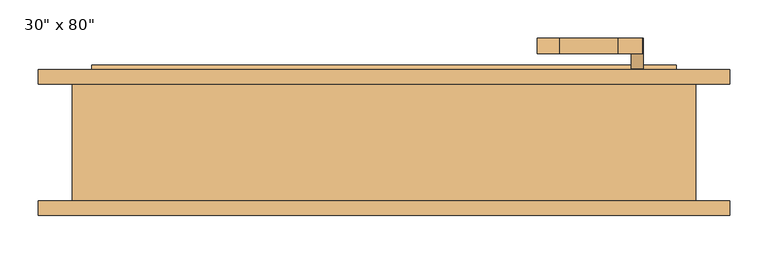
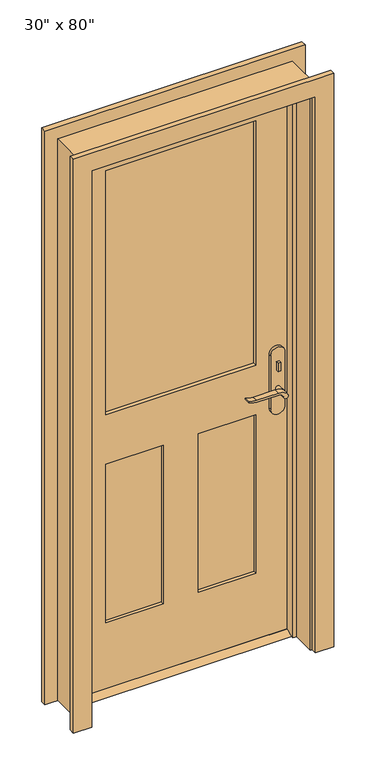
"""IFC4 building model written with IfcOpenShell, lengths in millimetres: door geometry."""

from ifc_helpers import new_model, si_unit, point, frame, frame_2d, origin, place, context, project, spatial, polyline, circle_curve, trimmed, segment, composite_curve, outline, extrude, faceted_brep, source, transform, mapped, element, save


def door_cdf9d6cc(model_context):
    return source(origin(), model_context, "Body", "SolidModel", [
        extrude(outline(polyline([(38.1, 12.7), (73.025, 12.7), (98.425, 0.0), (12.7, 0.0), (38.1, 12.7)])), frame((-381.0, 0.0, 0.0), z_axis=(1.0, 0.0, 0.0), x_axis=(0.0, 1.0, 0.0)), (0.0, 0.0, 1.0), 762.0),
        extrude(outline(polyline([(335.2, 18.1), (325.2, 18.1), (325.2, 28.1), (335.2, 28.1), (335.2, 18.1)])), frame((0.0, 0.0, 981.9), z_axis=(0.0, 0.0, 1.0), x_axis=(1.0, 0.0, 0.0)), (0.0, 0.0, 1.0), 30.0),
        extrude(outline(composite_curve([segment(trimmed(circle_curve(frame_2d((996.9, 330.2)), 8.0), [point((996.9, 322.2))], [point((996.9, 338.2))], False, "CARTESIAN"), True, "CONTINUOUS"), segment(trimmed(circle_curve(frame_2d((996.9, 330.2)), 8.0), [point((996.9, 338.2))], [point((996.9, 322.2))], False, "CARTESIAN"), True, "CONTINUOUS")], self_intersect=False)), frame((0.0, 83.025, 0.0), z_axis=(0.0, 1.0, 0.0), x_axis=(0.0, 0.0, 1.0)), (0.0, 0.0, 1.0), 10.0),
        extrude(outline(composite_curve([segment(trimmed(circle_curve(frame_2d((897.1555521, 306.5324871)), 37.2832219), [point((919.0523287, 336.7081363))], [point((934.4, 304.8325667))], False, "CARTESIAN"), True, "CONTINUOUS"), segment(polyline([(934.4, 304.8325667), (934.4, 228.5564091)]), True, "CONTINUOUS"), segment(trimmed(circle_curve(frame_2d((1017.6850638, 228.6227909)), 83.2850902), [point((934.4, 228.5564091))], [point((939.4, 200.2))], True, "CARTESIAN"), True, "CONTINUOUS"), segment(polyline([(939.4, 200.2), (936.6135558, 200.2)]), True, "CONTINUOUS"), segment(trimmed(circle_curve(frame_2d((986.6709207, 232.1396612)), 59.3791355), [point((936.6135558, 200.2))], [point((927.4, 228.5564091))], False, "CARTESIAN"), True, "CONTINUOUS"), segment(polyline([(927.4, 228.5564091), (927.4, 304.8138099)]), True, "CONTINUOUS"), segment(trimmed(circle_curve(frame_2d((909.2738613, 304.8138099)), 18.1261387), [point((927.4, 304.8138099))], [point((914.4, 322.2))], True, "CARTESIAN"), True, "CONTINUOUS"), segment(trimmed(circle_curve(frame_2d((914.4, 330.2)), 8.0), [point((914.4, 322.2))], [point((919.0523287, 336.7081363))], False, "CARTESIAN"), True, "CONTINUOUS")], self_intersect=False)), frame((0.0, -21.9, 0.0), z_axis=(0.0, 1.0, 0.0), x_axis=(0.0, 0.0, 1.0)), (0.0, 0.0, 1.0), 20.0),
        extrude(outline(composite_curve([segment(trimmed(circle_curve(frame_2d((914.4, 330.2)), 8.0), [point((914.3999903, 322.2))], [point((919.0523287, 336.7081363))], False, "CARTESIAN"), True, "CONTINUOUS"), segment(trimmed(circle_curve(frame_2d((897.1555521, 306.5324871)), 37.2832219), [point((919.0523287, 336.7081363))], [point((934.4, 304.8325667))], False, "CARTESIAN"), True, "CONTINUOUS"), segment(polyline([(934.4, 304.8325667), (934.4, 228.5564091)]), True, "CONTINUOUS"), segment(trimmed(circle_curve(frame_2d((1017.6850638, 228.6227909)), 83.2850902), [point((934.4, 228.5564091))], [point((939.4, 200.2))], True, "CARTESIAN"), True, "CONTINUOUS"), segment(polyline([(939.4, 200.2), (936.6135558, 200.2)]), True, "CONTINUOUS"), segment(trimmed(circle_curve(frame_2d((986.6709207, 232.1396612)), 59.3791355), [point((936.6135558, 200.2))], [point((927.4, 228.5564091))], False, "CARTESIAN"), True, "CONTINUOUS"), segment(polyline([(927.4, 228.5564091), (927.4, 304.8138122)]), True, "CONTINUOUS"), segment(trimmed(circle_curve(frame_2d((909.2738682, 304.8138122)), 18.1261318), [point((927.4, 304.8138122))], [point((914.3999903, 322.2))], True, "CARTESIAN"), True, "CONTINUOUS")], self_intersect=False)), frame((0.0, 113.025, 0.0), z_axis=(0.0, 1.0, 0.0), x_axis=(0.0, 0.0, 1.0)), (0.0, 0.0, 1.0), 20.0),
        extrude(outline(composite_curve([segment(trimmed(circle_curve(frame_2d((914.4, 330.2)), 8.0), [point((914.4, 322.2))], [point((914.4, 338.2))], False, "CARTESIAN"), True, "CONTINUOUS"), segment(trimmed(circle_curve(frame_2d((914.4, 330.2)), 8.0), [point((914.4, 338.2))], [point((914.4, 322.2))], False, "CARTESIAN"), True, "CONTINUOUS")], self_intersect=False)), frame((0.0, -1.9, 0.0), z_axis=(0.0, 1.0, 0.0), x_axis=(0.0, 0.0, 1.0)), (0.0, 0.0, 1.0), 30.0),
        extrude(outline(composite_curve([segment(trimmed(circle_curve(frame_2d((914.4, 330.2)), 8.0), [point((914.4, 322.2))], [point((914.4, 338.2))], False, "CARTESIAN"), True, "CONTINUOUS"), segment(trimmed(circle_curve(frame_2d((914.4, 330.2)), 8.0), [point((914.4, 338.2))], [point((914.4, 322.2))], False, "CARTESIAN"), True, "CONTINUOUS")], self_intersect=False)), frame((0.0, 83.025, 0.0), z_axis=(0.0, 1.0, 0.0), x_axis=(0.0, 0.0, 1.0)), (0.0, 0.0, 1.0), 30.0),
        extrude(outline(composite_curve([segment(polyline([(844.4, 355.2), (1039.4, 355.2)]), True, "CONTINUOUS"), segment(trimmed(circle_curve(frame_2d((1039.4, 330.2)), 25.0), [point((1039.4, 355.2))], [point((1039.4, 305.2))], False, "CARTESIAN"), True, "CONTINUOUS"), segment(polyline([(1039.4, 305.2), (844.4, 305.2)]), True, "CONTINUOUS"), segment(trimmed(circle_curve(frame_2d((844.4, 330.2)), 25.0), [point((844.4, 305.2))], [point((844.4, 355.2))], False, "CARTESIAN"), True, "CONTINUOUS")], self_intersect=False)), frame((0.0, 28.1, 0.0), z_axis=(0.0, 1.0, 0.0), x_axis=(0.0, 0.0, 1.0)), (0.0, 0.0, 1.0), 10.0),
        extrude(outline(composite_curve([segment(polyline([(844.4, 355.2), (1039.4, 355.2)]), True, "CONTINUOUS"), segment(trimmed(circle_curve(frame_2d((1039.4, 330.2)), 25.0), [point((1039.4, 355.2))], [point((1039.4, 305.2))], False, "CARTESIAN"), True, "CONTINUOUS"), segment(polyline([(1039.4, 305.2), (844.4, 305.2)]), True, "CONTINUOUS"), segment(trimmed(circle_curve(frame_2d((844.4, 330.2)), 25.0), [point((844.4, 305.2))], [point((844.4, 355.2))], False, "CARTESIAN"), True, "CONTINUOUS")], self_intersect=False)), frame((0.0, 73.025, 0.0), z_axis=(0.0, 1.0, 0.0), x_axis=(0.0, 0.0, 1.0)), (0.0, 0.0, 1.0), 10.0),
        extrude(outline(polyline([(2032.0, -381.0), (12.7, -381.0), (12.7, 381.0), (2032.0, 381.0), (2032.0, -381.0)]), holes=[polyline([(1016.0, -260.35), (1911.35, -260.35), (1911.35, 260.35), (1016.0, 260.35), (1016.0, -260.35)]), polyline([(835.025, -60.325), (254.0, -60.325), (254.0, -260.35), (835.025, -260.35), (835.025, -60.325)]), polyline([(835.025, 260.35), (254.0, 260.35), (254.0, 60.325), (835.025, 60.325), (835.025, 260.35)])]), frame((0.0, 38.1, 0.0), z_axis=(0.0, 1.0, 0.0), x_axis=(0.0, 0.0, 1.0)), (0.0, 0.0, 1.0), 34.925),
        faceted_brep([(406.4, 73.025, 0.0), (406.4, -79.375, 0.0), (381.0, -79.375, 0.0), (381.0, 3.175, 0.0), (368.3, 3.175, 0.0), (368.3, 38.1, 0.0), (381.0, 38.1, 0.0), (381.0, 73.025, 0.0), (406.4, 73.025, 2057.4), (406.4, -79.375, 2057.4), (-406.4, -79.375, 2057.4), (-406.4, -79.375, 0.0), (-381.0, -79.375, 0.0), (-381.0, -79.375, 2032.0), (381.0, -79.375, 2032.0), (381.0, 3.175, 2032.0), (-381.0, 3.175, 2032.0), (-381.0, 3.175, 0.0), (-368.3, 3.175, 0.0), (-368.3, 3.175, 2019.3), (368.3, 3.175, 2019.3), (368.3, 38.1, 2019.3), (-368.3, 38.1, 2019.3), (-368.3, 38.1, 0.0), (-381.0, 38.1, 0.0), (-381.0, 38.1, 2032.0), (381.0, 38.1, 2032.0), (381.0, 73.025, 2032.0), (-381.0, 73.025, 2032.0), (-381.0, 73.025, 0.0), (-406.4, 73.025, 0.0), (-406.4, 73.025, 2057.4)], [[[0, 1, 2, 3, 4, 5, 6, 7]], [[1, 0, 8, 9]], [[2, 1, 9, 10, 11, 12, 13, 14]], [[3, 2, 14, 15]], [[4, 3, 15, 16, 17, 18, 19, 20]], [[5, 4, 20, 21]], [[6, 5, 21, 22, 23, 24, 25, 26]], [[7, 6, 26, 27]], [[0, 7, 27, 28, 29, 30, 31, 8]], [[9, 8, 31, 10]], [[15, 14, 13, 16]], [[21, 20, 19, 22]], [[27, 26, 25, 28]], [[30, 29, 24, 23, 18, 17, 12, 11]], [[10, 31, 30, 11]], [[16, 13, 12, 17]], [[22, 19, 18, 23]], [[28, 25, 24, 29]]]),
        extrude(outline(polyline([(-60.325, 49.7416667), (-260.35, 49.7416667), (-260.35, 61.3833333), (-60.325, 61.3833333), (-60.325, 49.7416667)])), frame((0.0, 0.0, 254.0), z_axis=(0.0, 0.0, 1.0), x_axis=(1.0, 0.0, 0.0)), (0.0, 0.0, 1.0), 581.025),
        extrude(outline(polyline([(260.35, 49.7416667), (60.325, 49.7416667), (60.325, 61.3833333), (260.35, 61.3833333), (260.35, 49.7416667)])), frame((0.0, 0.0, 254.0), z_axis=(0.0, 0.0, 1.0), x_axis=(1.0, 0.0, 0.0)), (0.0, 0.0, 1.0), 581.025),
        extrude(outline(polyline([(260.35, 52.07), (-260.35, 52.07), (-260.35, 59.055), (260.35, 59.055), (260.35, 52.07)])), frame((0.0, 0.0, 1016.0), z_axis=(0.0, 0.0, 1.0), x_axis=(1.0, 0.0, 0.0)), (0.0, 0.0, 1.0), 895.35),
        extrude(outline(polyline([(0.0, -450.85), (0.0, -387.35), (2038.35, -387.35), (2038.35, 387.35), (0.0, 387.35), (0.0, 450.85), (2101.85, 450.85), (2101.85, -450.85), (0.0, -450.85)])), frame((0.0, -98.425, 0.0), z_axis=(0.0, 1.0, 0.0), x_axis=(0.0, 0.0, 1.0)), (0.0, 0.0, 1.0), 19.05),
        extrude(outline(polyline([(0.0, -450.85), (0.0, -387.35), (2038.35, -387.35), (2038.35, 387.35), (0.0, 387.35), (0.0, 450.85), (2101.85, 450.85), (2101.85, -450.85), (0.0, -450.85)])), frame((0.0, 73.025, 0.0), z_axis=(0.0, 1.0, 0.0), x_axis=(0.0, 0.0, 1.0)), (0.0, 0.0, 1.0), 19.05),
    ])


if __name__ == "__main__":
    model = new_model("IFC4")
    model_context = context("Model", 3, world=origin())
    ifc_project = project(units=[si_unit("LENGTHUNIT", "METRE", prefix="MILLI")], contexts=[model_context])
    site = spatial("IfcSite", under=ifc_project)
    building = spatial("IfcBuilding", under=site)
    placement = place(None, origin())
    door_shape = door_cdf9d6cc(model_context)
    element("IfcDoor", 1, ObjectType="30\" x 80\"", at=placement, inside=building, context=model_context, shape_type="MappedRepresentation", body=[
        mapped(door_shape, transform((0.0, 0.0, 0.0), x_axis=(1.0, 0.0, 0.0), y_axis=(0.0, 1.0, 0.0), z_axis=(0.0, 0.0, 1.0))),
    ])
    save(model, "model.ifc")

# Revit data of these elements
# Type "30\" x 80\""
#   Type Mark = "8"
#   Assembly Code = "B2030100"
#   Analytic Construction = "French door, wood frame with single glass"
#   Top Rail = 0' - 4 3/4"
#   Threshold Offset [instance default] = 0' - 0 1/2"
#   Thickness = 0' - 1 3/8"
#   Thermal Resistance (R) = 1.0696 (h·ft²·°F)/BTU
#   Swing Angle [instance default] = 90.00°
#   Stiles = 0' - 4 3/4"
#   Rough Width = 2' - 8"
#   Rough Height = 6' - 9"
#   Lock Rail = 0' - 7 1/8"
#   Height = 6' - 8"
#   Width = 2' - 6"
#   Heat Transfer Coefficient (U) = 0.9350 BTU/(h·ft²·°F)
#   Door Offset [instance default] = 0' - 0"
#   Bottom Rail = 0' - 9 1/2"
#   Threshold [instance default] = yes
#   Function = 1
#   Exterior Trim [instance default] = yes
#   Trim Material = Cherry
#   Threshold Material = Cherry
#   Panel Material = Cherry
#   Glazing = Glass
#   Frame Material = Cherry
#   Door Handle Material = Aluminum
#   Visual Light Transmittance = 0
#   Solar Heat Gain Coefficient = 0
#   Wall Closure = (empty or 0)
#   Construction Type = (empty or 0)
# Element 1 (IfcDoor, "30\" x 80\"")
#   Materials on its faces: "Cherry", "Aluminum", "Glass"
# Materials
#   "Cherry": class "Wood", colour RGB 226 177 128, transparency 0, Description = "Prunus Serotina", Cost = 0
#   "Glass": class "Glass", colour RGB 0 128 192, transparency 0.75, Description = "Soda Lime Glass", Cost = 0
#   "Aluminum": class "Metal", colour RGB 247 247 247, transparency 0, Description = "Aluminum 6061", Cost = 0
